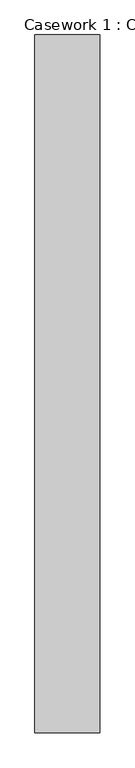
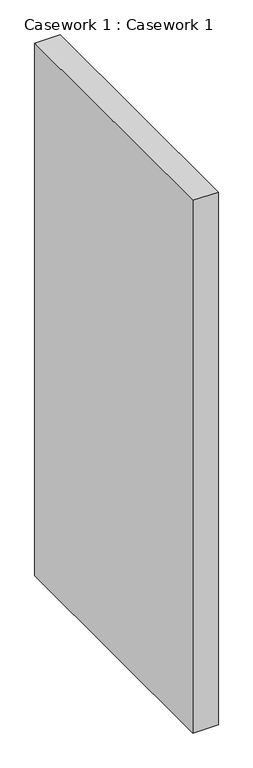
"""IFC4 building model written with IfcOpenShell, lengths in millimetres: furniture geometry, Casework 1 : Casework 1."""

from ifc_helpers import new_model, si_unit, frame, origin, place, context, project, spatial, polyline, outline, extrude, source, transform, mapped, element, save


def casework_1_casework_1_07494d98(model_context):
    return source(origin(), model_context, "Body", "SweptSolid", [
        extrude(outline(polyline([(-16201.8794706, -1359.9833944), (-16201.8794706, -132.2741596), (-16087.5794706, -132.2741596), (-16087.5794706, -1359.9833944), (-16201.8794706, -1359.9833944)])), frame((0.0, 0.0, 3150.0), z_axis=(0.0, 0.0, 1.0), x_axis=(1.0, 0.0, 0.0)), (0.0, 0.0, 1.0), 2523.2452345),
    ])


if __name__ == "__main__":
    model = new_model("IFC4")
    model_context = context("Model", 3, world=origin())
    ifc_project = project(units=[si_unit("LENGTHUNIT", "METRE", prefix="MILLI")], contexts=[model_context])
    site = spatial("IfcSite", under=ifc_project)
    building = spatial("IfcBuilding", under=site)
    placement = place(None, origin())
    casework_1_casework_1_shape = casework_1_casework_1_07494d98(model_context)
    element("IfcFurniture", 1, ObjectType="Casework 1 : Casework 1", at=placement, inside=building, context=model_context, shape_type="MappedRepresentation", body=[
        mapped(casework_1_casework_1_shape, transform((0.0, 0.0, 0.0), x_axis=(1.0, 0.0, 0.0), y_axis=(0.0, 1.0, 0.0), z_axis=(0.0, 0.0, 1.0))),
    ])
    save(model, "model.ifc")
